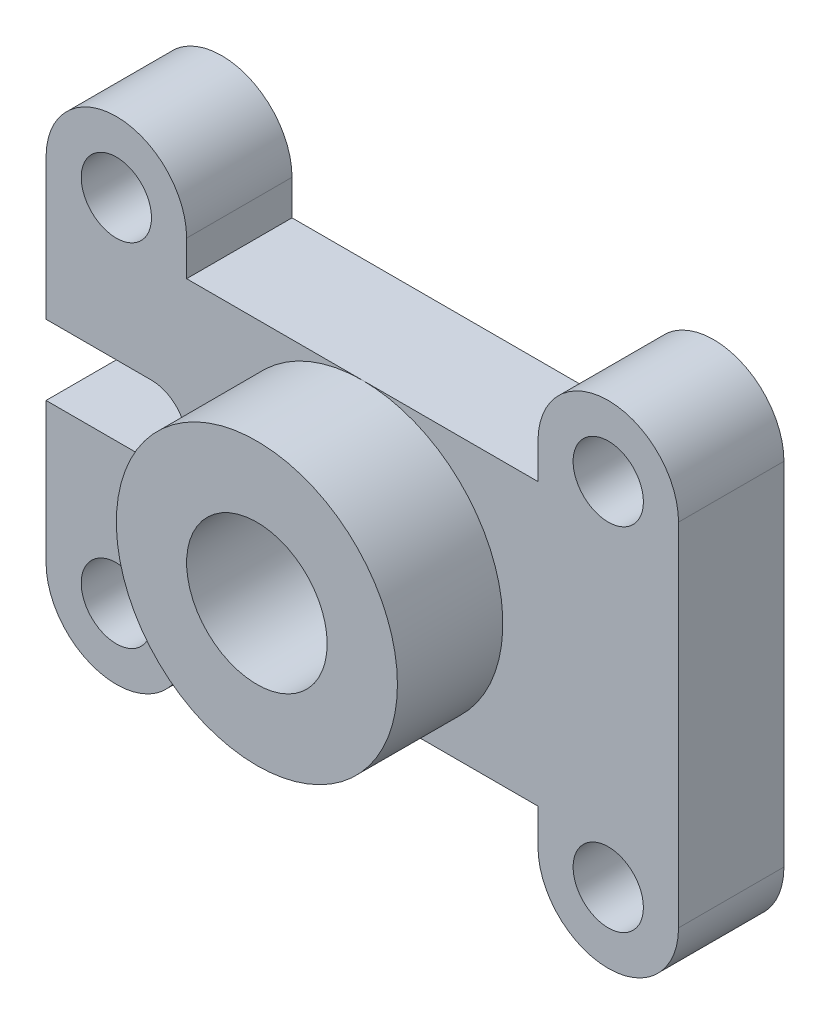
ISO-10303-21;
HEADER;
FILE_DESCRIPTION(('STEP AP214'),'2;1');
FILE_NAME('part.step','',(''),(''),'','','');
FILE_SCHEMA(('AUTOMOTIVE_DESIGN { 1 0 10303 214 1 1 1 1 }'));
ENDSEC;
DATA;
#1=APPLICATION_CONTEXT('core data for automotive mechanical design processes');
#2=APPLICATION_PROTOCOL_DEFINITION('international standard','automotive_design',2000,#1);
#3=PRODUCT_CONTEXT('',#1,'mechanical');
#4=PRODUCT('Part','Part','',(#3));
#5=PRODUCT_RELATED_PRODUCT_CATEGORY('part','',(#4));
#6=PRODUCT_DEFINITION_FORMATION('','',#4);
#7=PRODUCT_DEFINITION_CONTEXT('part definition',#1,'design');
#8=PRODUCT_DEFINITION('design','',#6,#7);
#9=PRODUCT_DEFINITION_SHAPE('','',#8);
#10=(LENGTH_UNIT() NAMED_UNIT(*) SI_UNIT(.MILLI.,.METRE.));
#11=(NAMED_UNIT(*) PLANE_ANGLE_UNIT() SI_UNIT($,.RADIAN.));
#12=(NAMED_UNIT(*) SI_UNIT($,.STERADIAN.) SOLID_ANGLE_UNIT());
#13=UNCERTAINTY_MEASURE_WITH_UNIT(LENGTH_MEASURE(1.E-05),#10,'distance_accuracy_value','');
#14=(GEOMETRIC_REPRESENTATION_CONTEXT(3) GLOBAL_UNCERTAINTY_ASSIGNED_CONTEXT((#13)) GLOBAL_UNIT_ASSIGNED_CONTEXT((#10,
#11,#12)) REPRESENTATION_CONTEXT('',''));
#15=CARTESIAN_POINT('',(0.,0.,0.));
#16=DIRECTION('',(0.,0.,1.));
#17=DIRECTION('',(1.,0.,0.));
#18=AXIS2_PLACEMENT_3D('',#15,#16,#17);
#19=CARTESIAN_POINT('',(-10.,0.,15.));
#20=DIRECTION('',(1.,0.,0.));
#21=DIRECTION('',(0.,1.,0.));
#22=AXIS2_PLACEMENT_3D('',#19,#20,#21);
#23=PLANE('',#22);
#24=DIRECTION('',(0.,-1.,0.));
#25=VECTOR('',#24,1.);
#26=CARTESIAN_POINT('',(-10.,0.,15.));
#27=LINE('',#26,#25);
#28=CARTESIAN_POINT('',(-10.,20.,15.));
#29=VERTEX_POINT('',#28);
#30=CARTESIAN_POINT('',(-10.,0.,15.));
#31=VERTEX_POINT('',#30);
#32=EDGE_CURVE('E262',#29,#31,#27,.T.);
#33=ORIENTED_EDGE('',*,*,#32,.F.);
#34=DIRECTION('',(0.,0.,1.));
#35=VECTOR('',#34,1.);
#36=CARTESIAN_POINT('',(-10.,20.,0.));
#37=LINE('',#36,#35);
#38=CARTESIAN_POINT('',(-10.,20.,0.));
#39=VERTEX_POINT('',#38);
#40=EDGE_CURVE('E197',#39,#29,#37,.T.);
#41=ORIENTED_EDGE('',*,*,#40,.F.);
#42=DIRECTION('',(0.,-1.,0.));
#43=VECTOR('',#42,1.);
#44=CARTESIAN_POINT('',(-10.,0.,0.));
#45=LINE('',#44,#43);
#46=CARTESIAN_POINT('',(-10.,0.,0.));
#47=VERTEX_POINT('',#46);
#48=EDGE_CURVE('E289',#39,#47,#45,.T.);
#49=ORIENTED_EDGE('',*,*,#48,.T.);
#50=DIRECTION('',(0.,0.,-1.));
#51=VECTOR('',#50,1.);
#52=CARTESIAN_POINT('',(-10.,0.,15.));
#53=LINE('',#52,#51);
#54=EDGE_CURVE('E322',#31,#47,#53,.T.);
#55=ORIENTED_EDGE('',*,*,#54,.F.);
#56=EDGE_LOOP('',(#33,#41,#49,#55));
#57=FACE_BOUND('',#56,.T.);
#58=ADVANCED_FACE('F50',(#57),#23,.F.);
#59=CARTESIAN_POINT('',(0.,0.,15.));
#60=DIRECTION('',(0.,0.,1.));
#61=DIRECTION('',(1.,0.,0.));
#62=AXIS2_PLACEMENT_3D('',#59,#60,#61);
#63=PLANE('',#62);
#64=DIRECTION('',(1.,0.,0.));
#65=VECTOR('',#64,1.);
#66=CARTESIAN_POINT('',(5.,20.,15.));
#67=LINE('',#66,#65);
#68=CARTESIAN_POINT('',(5.,20.,15.));
#69=VERTEX_POINT('',#68);
#70=EDGE_CURVE('E190',#29,#69,#67,.T.);
#71=ORIENTED_EDGE('',*,*,#70,.F.);
#72=ORIENTED_EDGE('',*,*,#32,.T.);
#73=CARTESIAN_POINT('',(0.,0.,15.));
#74=DIRECTION('',(0.,0.,1.));
#75=DIRECTION('',(1.,0.,0.));
#76=AXIS2_PLACEMENT_3D('',#73,#74,#75);
#77=CIRCLE('',#76,10.);
#78=CARTESIAN_POINT('',(10.,0.,15.));
#79=VERTEX_POINT('',#78);
#80=EDGE_CURVE('E268',#31,#79,#77,.T.);
#81=ORIENTED_EDGE('',*,*,#80,.T.);
#82=DIRECTION('',(0.,1.,0.));
#83=VECTOR('',#82,1.);
#84=CARTESIAN_POINT('',(10.,0.,15.));
#85=LINE('',#84,#83);
#86=CARTESIAN_POINT('',(10.,5.,15.));
#87=VERTEX_POINT('',#86);
#88=EDGE_CURVE('E269',#79,#87,#85,.T.);
#89=ORIENTED_EDGE('',*,*,#88,.T.);
#90=DIRECTION('',(-1.,0.,0.));
#91=VECTOR('',#90,1.);
#92=CARTESIAN_POINT('',(10.,5.,15.));
#93=LINE('',#92,#91);
#94=CARTESIAN_POINT('',(35.,5.00000000000001,15.));
#95=VERTEX_POINT('',#94);
#96=EDGE_CURVE('E245',#95,#87,#93,.T.);
#97=ORIENTED_EDGE('',*,*,#96,.F.);
#98=CARTESIAN_POINT('',(35.,25.,15.));
#99=DIRECTION('',(0.,0.,1.));
#100=DIRECTION('',(1.,0.,0.));
#101=AXIS2_PLACEMENT_3D('',#98,#99,#100);
#102=CIRCLE('',#101,20.);
#103=CARTESIAN_POINT('',(35.,45.,15.));
#104=VERTEX_POINT('',#103);
#105=EDGE_CURVE('E60',#104,#95,#102,.T.);
#106=ORIENTED_EDGE('',*,*,#105,.F.);
#107=DIRECTION('',(1.,0.,0.));
#108=VECTOR('',#107,1.);
#109=CARTESIAN_POINT('',(60.,45.,15.));
#110=LINE('',#109,#108);
#111=CARTESIAN_POINT('',(10.,45.,15.));
#112=VERTEX_POINT('',#111);
#113=EDGE_CURVE('E249',#112,#104,#110,.T.);
#114=ORIENTED_EDGE('',*,*,#113,.F.);
#115=DIRECTION('',(0.,1.,0.));
#116=VECTOR('',#115,1.);
#117=CARTESIAN_POINT('',(10.,0.,15.));
#118=LINE('',#117,#116);
#119=CARTESIAN_POINT('',(10.,50.,15.));
#120=VERTEX_POINT('',#119);
#121=EDGE_CURVE('E256',#112,#120,#118,.T.);
#122=ORIENTED_EDGE('',*,*,#121,.T.);
#123=CARTESIAN_POINT('',(0.,50.,15.));
#124=DIRECTION('',(0.,0.,1.));
#125=DIRECTION('',(1.,0.,0.));
#126=AXIS2_PLACEMENT_3D('',#123,#124,#125);
#127=CIRCLE('',#126,10.);
#128=CARTESIAN_POINT('',(-10.,50.,15.));
#129=VERTEX_POINT('',#128);
#130=EDGE_CURVE('E261',#120,#129,#127,.T.);
#131=ORIENTED_EDGE('',*,*,#130,.T.);
#132=CARTESIAN_POINT('',(-10.,30.,15.));
#133=VERTEX_POINT('',#132);
#134=EDGE_CURVE('E264',#129,#133,#27,.T.);
#135=ORIENTED_EDGE('',*,*,#134,.T.);
#136=DIRECTION('',(-1.,0.,0.));
#137=VECTOR('',#136,1.);
#138=CARTESIAN_POINT('',(5.,30.,15.));
#139=LINE('',#138,#137);
#140=CARTESIAN_POINT('',(5.,30.,15.));
#141=VERTEX_POINT('',#140);
#142=EDGE_CURVE('E188',#141,#133,#139,.T.);
#143=ORIENTED_EDGE('',*,*,#142,.F.);
#144=CARTESIAN_POINT('',(5.,25.,15.));
#145=DIRECTION('',(0.,0.,1.));
#146=DIRECTION('',(1.,0.,0.));
#147=AXIS2_PLACEMENT_3D('',#144,#145,#146);
#148=CIRCLE('',#147,5.);
#149=EDGE_CURVE('E174',#69,#141,#148,.T.);
#150=ORIENTED_EDGE('',*,*,#149,.F.);
#151=EDGE_LOOP('',(#71,#72,#81,#89,#97,#106,#114,#122,#131,#135,#143,#150));
#152=FACE_BOUND('',#151,.T.);
#153=CARTESIAN_POINT('',(0.,49.9999999999999,15.));
#154=DIRECTION('',(0.,0.,1.));
#155=DIRECTION('',(1.,0.,0.));
#156=AXIS2_PLACEMENT_3D('',#153,#154,#155);
#157=CIRCLE('',#156,5.);
#158=CARTESIAN_POINT('',(5.,49.9999999999999,15.));
#159=VERTEX_POINT('',#158);
#160=EDGE_CURVE('E198',#159,#159,#157,.T.);
#161=ORIENTED_EDGE('',*,*,#160,.F.);
#162=EDGE_LOOP('',(#161));
#163=FACE_BOUND('',#162,.T.);
#164=CARTESIAN_POINT('',(0.,0.,15.));
#165=DIRECTION('',(0.,0.,1.));
#166=DIRECTION('',(1.,0.,0.));
#167=AXIS2_PLACEMENT_3D('',#164,#165,#166);
#168=CIRCLE('',#167,5.);
#169=CARTESIAN_POINT('',(5.,0.,15.));
#170=VERTEX_POINT('',#169);
#171=EDGE_CURVE('E215',#170,#170,#168,.T.);
#172=ORIENTED_EDGE('',*,*,#171,.F.);
#173=EDGE_LOOP('',(#172));
#174=FACE_BOUND('',#173,.T.);
#175=ADVANCED_FACE('F342',(#152,#163,#174),#63,.T.);
#176=CARTESIAN_POINT('',(10.,0.,15.));
#177=DIRECTION('',(-1.,0.,0.));
#178=DIRECTION('',(0.,0.,1.));
#179=AXIS2_PLACEMENT_3D('',#176,#177,#178);
#180=PLANE('',#179);
#181=DIRECTION('',(0.,0.,-1.));
#182=VECTOR('',#181,1.);
#183=CARTESIAN_POINT('',(10.,5.,0.));
#184=LINE('',#183,#182);
#185=CARTESIAN_POINT('',(10.,5.,0.));
#186=VERTEX_POINT('',#185);
#187=EDGE_CURVE('E231',#87,#186,#184,.T.);
#188=ORIENTED_EDGE('',*,*,#187,.F.);
#189=ORIENTED_EDGE('',*,*,#88,.F.);
#190=DIRECTION('',(0.,0.,-1.));
#191=VECTOR('',#190,1.);
#192=CARTESIAN_POINT('',(10.,0.,15.));
#193=LINE('',#192,#191);
#194=CARTESIAN_POINT('',(10.,0.,0.));
#195=VERTEX_POINT('',#194);
#196=EDGE_CURVE('E319',#79,#195,#193,.T.);
#197=ORIENTED_EDGE('',*,*,#196,.T.);
#198=DIRECTION('',(0.,1.,0.));
#199=VECTOR('',#198,1.);
#200=CARTESIAN_POINT('',(10.,0.,0.));
#201=LINE('',#200,#199);
#202=EDGE_CURVE('E294',#195,#186,#201,.T.);
#203=ORIENTED_EDGE('',*,*,#202,.T.);
#204=EDGE_LOOP('',(#188,#189,#197,#203));
#205=FACE_BOUND('',#204,.T.);
#206=ADVANCED_FACE('F391',(#205),#180,.F.);
#207=CARTESIAN_POINT('',(60.,0.,15.));
#208=DIRECTION('',(-1.,0.,0.));
#209=DIRECTION('',(0.,0.,1.));
#210=AXIS2_PLACEMENT_3D('',#207,#208,#209);
#211=PLANE('',#210);
#212=DIRECTION('',(0.,1.,0.));
#213=VECTOR('',#212,1.);
#214=CARTESIAN_POINT('',(60.,0.,15.));
#215=LINE('',#214,#213);
#216=CARTESIAN_POINT('',(60.,0.,15.));
#217=VERTEX_POINT('',#216);
#218=CARTESIAN_POINT('',(60.,5.00000000000001,15.));
#219=VERTEX_POINT('',#218);
#220=EDGE_CURVE('E271',#217,#219,#215,.T.);
#221=ORIENTED_EDGE('',*,*,#220,.T.);
#222=DIRECTION('',(0.,0.,1.));
#223=VECTOR('',#222,1.);
#224=CARTESIAN_POINT('',(60.,5.00000000000001,15.));
#225=LINE('',#224,#223);
#226=CARTESIAN_POINT('',(60.,5.00000000000001,0.));
#227=VERTEX_POINT('',#226);
#228=EDGE_CURVE('E239',#227,#219,#225,.T.);
#229=ORIENTED_EDGE('',*,*,#228,.F.);
#230=DIRECTION('',(0.,1.,0.));
#231=VECTOR('',#230,1.);
#232=CARTESIAN_POINT('',(60.,0.,0.));
#233=LINE('',#232,#231);
#234=CARTESIAN_POINT('',(60.,0.,0.));
#235=VERTEX_POINT('',#234);
#236=EDGE_CURVE('E296',#235,#227,#233,.T.);
#237=ORIENTED_EDGE('',*,*,#236,.F.);
#238=DIRECTION('',(0.,0.,-1.));
#239=VECTOR('',#238,1.);
#240=CARTESIAN_POINT('',(60.,0.,15.));
#241=LINE('',#240,#239);
#242=EDGE_CURVE('E317',#217,#235,#241,.T.);
#243=ORIENTED_EDGE('',*,*,#242,.F.);
#244=EDGE_LOOP('',(#221,#229,#237,#243));
#245=FACE_BOUND('',#244,.T.);
#246=ADVANCED_FACE('F366',(#245),#211,.T.);
#247=CARTESIAN_POINT('',(10.,0.,15.));
#248=DIRECTION('',(-1.,0.,0.));
#249=DIRECTION('',(0.,0.,1.));
#250=AXIS2_PLACEMENT_3D('',#247,#248,#249);
#251=PLANE('',#250);
#252=DIRECTION('',(0.,0.,1.));
#253=VECTOR('',#252,1.);
#254=CARTESIAN_POINT('',(10.,45.,15.));
#255=LINE('',#254,#253);
#256=CARTESIAN_POINT('',(10.,45.,0.));
#257=VERTEX_POINT('',#256);
#258=EDGE_CURVE('E246',#257,#112,#255,.T.);
#259=ORIENTED_EDGE('',*,*,#258,.F.);
#260=DIRECTION('',(0.,1.,0.));
#261=VECTOR('',#260,1.);
#262=CARTESIAN_POINT('',(10.,0.,0.));
#263=LINE('',#262,#261);
#264=CARTESIAN_POINT('',(10.,50.,0.));
#265=VERTEX_POINT('',#264);
#266=EDGE_CURVE('E259',#257,#265,#263,.T.);
#267=ORIENTED_EDGE('',*,*,#266,.T.);
#268=DIRECTION('',(0.,0.,-1.));
#269=VECTOR('',#268,1.);
#270=CARTESIAN_POINT('',(10.,50.,15.));
#271=LINE('',#270,#269);
#272=EDGE_CURVE('E51',#120,#265,#271,.T.);
#273=ORIENTED_EDGE('',*,*,#272,.F.);
#274=ORIENTED_EDGE('',*,*,#121,.F.);
#275=EDGE_LOOP('',(#259,#267,#273,#274));
#276=FACE_BOUND('',#275,.T.);
#277=ADVANCED_FACE('F47',(#276),#251,.F.);
#278=CARTESIAN_POINT('',(60.,0.,15.));
#279=DIRECTION('',(1.,0.,0.));
#280=DIRECTION('',(0.,0.,-1.));
#281=AXIS2_PLACEMENT_3D('',#278,#279,#280);
#282=PLANE('',#281);
#283=DIRECTION('',(0.,0.,-1.));
#284=VECTOR('',#283,1.);
#285=CARTESIAN_POINT('',(60.,45.,0.));
#286=LINE('',#285,#284);
#287=CARTESIAN_POINT('',(60.,45.,15.));
#288=VERTEX_POINT('',#287);
#289=CARTESIAN_POINT('',(60.,45.,0.));
#290=VERTEX_POINT('',#289);
#291=EDGE_CURVE('E255',#288,#290,#286,.T.);
#292=ORIENTED_EDGE('',*,*,#291,.F.);
#293=DIRECTION('',(0.,-1.,0.));
#294=VECTOR('',#293,1.);
#295=CARTESIAN_POINT('',(60.,0.,15.));
#296=LINE('',#295,#294);
#297=CARTESIAN_POINT('',(60.,50.,15.));
#298=VERTEX_POINT('',#297);
#299=EDGE_CURVE('E283',#298,#288,#296,.T.);
#300=ORIENTED_EDGE('',*,*,#299,.F.);
#301=DIRECTION('',(0.,0.,-1.));
#302=VECTOR('',#301,1.);
#303=CARTESIAN_POINT('',(60.,50.,15.));
#304=LINE('',#303,#302);
#305=CARTESIAN_POINT('',(60.,50.,0.));
#306=VERTEX_POINT('',#305);
#307=EDGE_CURVE('E286',#298,#306,#304,.T.);
#308=ORIENTED_EDGE('',*,*,#307,.T.);
#309=DIRECTION('',(0.,-1.,0.));
#310=VECTOR('',#309,1.);
#311=CARTESIAN_POINT('',(60.,0.,0.));
#312=LINE('',#311,#310);
#313=EDGE_CURVE('E265',#306,#290,#312,.T.);
#314=ORIENTED_EDGE('',*,*,#313,.T.);
#315=EDGE_LOOP('',(#292,#300,#308,#314));
#316=FACE_BOUND('',#315,.T.);
#317=ADVANCED_FACE('F351',(#316),#282,.F.);
#318=CARTESIAN_POINT('',(0.,50.,15.));
#319=DIRECTION('',(0.,0.,-1.));
#320=DIRECTION('',(-1.,0.,0.));
#321=AXIS2_PLACEMENT_3D('',#318,#319,#320);
#322=CYLINDRICAL_SURFACE('',#321,10.);
#323=CARTESIAN_POINT('',(0.,50.,0.));
#324=DIRECTION('',(0.,0.,1.));
#325=DIRECTION('',(1.,0.,0.));
#326=AXIS2_PLACEMENT_3D('',#323,#324,#325);
#327=CIRCLE('',#326,10.);
#328=CARTESIAN_POINT('',(-10.,50.,0.));
#329=VERTEX_POINT('',#328);
#330=EDGE_CURVE('E288',#265,#329,#327,.T.);
#331=ORIENTED_EDGE('',*,*,#330,.T.);
#332=DIRECTION('',(0.,0.,-1.));
#333=VECTOR('',#332,1.);
#334=CARTESIAN_POINT('',(-10.,50.,15.));
#335=LINE('',#334,#333);
#336=EDGE_CURVE('E324',#129,#329,#335,.T.);
#337=ORIENTED_EDGE('',*,*,#336,.F.);
#338=ORIENTED_EDGE('',*,*,#130,.F.);
#339=ORIENTED_EDGE('',*,*,#272,.T.);
#340=EDGE_LOOP('',(#331,#337,#338,#339));
#341=FACE_BOUND('',#340,.T.);
#342=ADVANCED_FACE('F335',(#341),#322,.T.);
#343=CARTESIAN_POINT('',(-10.,30.,0.));
#344=VERTEX_POINT('',#343);
#345=EDGE_CURVE('E293',#329,#344,#45,.T.);
#346=ORIENTED_EDGE('',*,*,#345,.T.);
#347=DIRECTION('',(0.,0.,1.));
#348=VECTOR('',#347,1.);
#349=CARTESIAN_POINT('',(-10.,30.,0.));
#350=LINE('',#349,#348);
#351=EDGE_CURVE('E61',#344,#133,#350,.T.);
#352=ORIENTED_EDGE('',*,*,#351,.T.);
#353=ORIENTED_EDGE('',*,*,#134,.F.);
#354=ORIENTED_EDGE('',*,*,#336,.T.);
#355=EDGE_LOOP('',(#346,#352,#353,#354));
#356=FACE_BOUND('',#355,.T.);
#357=ADVANCED_FACE('F336',(#356),#23,.F.);
#358=CARTESIAN_POINT('',(0.,0.,15.));
#359=DIRECTION('',(0.,0.,-1.));
#360=DIRECTION('',(-1.,0.,0.));
#361=AXIS2_PLACEMENT_3D('',#358,#359,#360);
#362=CYLINDRICAL_SURFACE('',#361,10.);
#363=CARTESIAN_POINT('',(0.,0.,0.));
#364=DIRECTION('',(0.,0.,1.));
#365=DIRECTION('',(1.,0.,0.));
#366=AXIS2_PLACEMENT_3D('',#363,#364,#365);
#367=CIRCLE('',#366,10.);
#368=EDGE_CURVE('E291',#47,#195,#367,.T.);
#369=ORIENTED_EDGE('',*,*,#368,.T.);
#370=ORIENTED_EDGE('',*,*,#196,.F.);
#371=ORIENTED_EDGE('',*,*,#80,.F.);
#372=ORIENTED_EDGE('',*,*,#54,.T.);
#373=EDGE_LOOP('',(#369,#370,#371,#372));
#374=FACE_BOUND('',#373,.T.);
#375=ADVANCED_FACE('F372',(#374),#362,.T.);
#376=CARTESIAN_POINT('',(70.,0.,15.));
#377=DIRECTION('',(0.,0.,-1.));
#378=DIRECTION('',(-1.,0.,0.));
#379=AXIS2_PLACEMENT_3D('',#376,#377,#378);
#380=CYLINDRICAL_SURFACE('',#379,10.);
#381=CARTESIAN_POINT('',(70.,0.,0.));
#382=DIRECTION('',(0.,0.,1.));
#383=DIRECTION('',(1.,0.,0.));
#384=AXIS2_PLACEMENT_3D('',#381,#382,#383);
#385=CIRCLE('',#384,10.);
#386=CARTESIAN_POINT('',(80.,0.,0.));
#387=VERTEX_POINT('',#386);
#388=EDGE_CURVE('E301',#235,#387,#385,.T.);
#389=ORIENTED_EDGE('',*,*,#388,.T.);
#390=DIRECTION('',(0.,0.,-1.));
#391=VECTOR('',#390,1.);
#392=CARTESIAN_POINT('',(80.,0.,15.));
#393=LINE('',#392,#391);
#394=CARTESIAN_POINT('',(80.,0.,15.));
#395=VERTEX_POINT('',#394);
#396=EDGE_CURVE('E313',#395,#387,#393,.T.);
#397=ORIENTED_EDGE('',*,*,#396,.F.);
#398=CARTESIAN_POINT('',(70.,0.,15.));
#399=DIRECTION('',(0.,0.,1.));
#400=DIRECTION('',(1.,0.,0.));
#401=AXIS2_PLACEMENT_3D('',#398,#399,#400);
#402=CIRCLE('',#401,10.);
#403=EDGE_CURVE('E277',#217,#395,#402,.T.);
#404=ORIENTED_EDGE('',*,*,#403,.F.);
#405=ORIENTED_EDGE('',*,*,#242,.T.);
#406=EDGE_LOOP('',(#389,#397,#404,#405));
#407=FACE_BOUND('',#406,.T.);
#408=ADVANCED_FACE('F375',(#407),#380,.T.);
#409=CARTESIAN_POINT('',(80.,0.,15.));
#410=DIRECTION('',(1.,0.,0.));
#411=DIRECTION('',(0.,0.,-1.));
#412=AXIS2_PLACEMENT_3D('',#409,#410,#411);
#413=PLANE('',#412);
#414=DIRECTION('',(0.,-1.,0.));
#415=VECTOR('',#414,1.);
#416=CARTESIAN_POINT('',(80.,0.,0.));
#417=LINE('',#416,#415);
#418=CARTESIAN_POINT('',(80.,50.,0.));
#419=VERTEX_POINT('',#418);
#420=EDGE_CURVE('E302',#419,#387,#417,.T.);
#421=ORIENTED_EDGE('',*,*,#420,.F.);
#422=DIRECTION('',(0.,0.,-1.));
#423=VECTOR('',#422,1.);
#424=CARTESIAN_POINT('',(80.,50.,15.));
#425=LINE('',#424,#423);
#426=CARTESIAN_POINT('',(80.,50.,15.));
#427=VERTEX_POINT('',#426);
#428=EDGE_CURVE('E315',#427,#419,#425,.T.);
#429=ORIENTED_EDGE('',*,*,#428,.F.);
#430=DIRECTION('',(0.,-1.,0.));
#431=VECTOR('',#430,1.);
#432=CARTESIAN_POINT('',(80.,0.,15.));
#433=LINE('',#432,#431);
#434=EDGE_CURVE('E279',#427,#395,#433,.T.);
#435=ORIENTED_EDGE('',*,*,#434,.T.);
#436=ORIENTED_EDGE('',*,*,#396,.T.);
#437=EDGE_LOOP('',(#421,#429,#435,#436));
#438=FACE_BOUND('',#437,.T.);
#439=ADVANCED_FACE('F360',(#438),#413,.T.);
#440=CARTESIAN_POINT('',(70.,50.,15.));
#441=DIRECTION('',(0.,0.,-1.));
#442=DIRECTION('',(-1.,0.,0.));
#443=AXIS2_PLACEMENT_3D('',#440,#441,#442);
#444=CYLINDRICAL_SURFACE('',#443,10.);
#445=CARTESIAN_POINT('',(70.,50.,0.));
#446=DIRECTION('',(0.,0.,1.));
#447=DIRECTION('',(1.,0.,0.));
#448=AXIS2_PLACEMENT_3D('',#445,#446,#447);
#449=CIRCLE('',#448,10.);
#450=EDGE_CURVE('E310',#419,#306,#449,.T.);
#451=ORIENTED_EDGE('',*,*,#450,.T.);
#452=ORIENTED_EDGE('',*,*,#307,.F.);
#453=CARTESIAN_POINT('',(70.,50.,15.));
#454=DIRECTION('',(0.,0.,1.));
#455=DIRECTION('',(1.,0.,0.));
#456=AXIS2_PLACEMENT_3D('',#453,#454,#455);
#457=CIRCLE('',#456,10.);
#458=EDGE_CURVE('E281',#427,#298,#457,.T.);
#459=ORIENTED_EDGE('',*,*,#458,.F.);
#460=ORIENTED_EDGE('',*,*,#428,.T.);
#461=EDGE_LOOP('',(#451,#452,#459,#460));
#462=FACE_BOUND('',#461,.T.);
#463=ADVANCED_FACE('F358',(#462),#444,.T.);
#464=CARTESIAN_POINT('',(70.,0.,15.));
#465=DIRECTION('',(0.,0.,1.));
#466=DIRECTION('',(1.,0.,0.));
#467=AXIS2_PLACEMENT_3D('',#464,#465,#466);
#468=CIRCLE('',#467,5.);
#469=CARTESIAN_POINT('',(75.,0.,15.));
#470=VERTEX_POINT('',#469);
#471=EDGE_CURVE('E207',#470,#470,#468,.T.);
#472=ORIENTED_EDGE('',*,*,#471,.F.);
#473=EDGE_LOOP('',(#472));
#474=FACE_BOUND('',#473,.T.);
#475=CARTESIAN_POINT('',(70.,50.,15.));
#476=DIRECTION('',(0.,0.,1.));
#477=DIRECTION('',(1.,0.,0.));
#478=AXIS2_PLACEMENT_3D('',#475,#476,#477);
#479=CIRCLE('',#478,5.00000000000001);
#480=CARTESIAN_POINT('',(75.,50.,15.));
#481=VERTEX_POINT('',#480);
#482=EDGE_CURVE('E204',#481,#481,#479,.T.);
#483=ORIENTED_EDGE('',*,*,#482,.F.);
#484=EDGE_LOOP('',(#483));
#485=FACE_BOUND('',#484,.T.);
#486=EDGE_CURVE('E11',#95,#104,#102,.T.);
#487=ORIENTED_EDGE('',*,*,#486,.F.);
#488=EDGE_CURVE('E243',#219,#95,#93,.T.);
#489=ORIENTED_EDGE('',*,*,#488,.F.);
#490=ORIENTED_EDGE('',*,*,#220,.F.);
#491=ORIENTED_EDGE('',*,*,#403,.T.);
#492=ORIENTED_EDGE('',*,*,#434,.F.);
#493=ORIENTED_EDGE('',*,*,#458,.T.);
#494=ORIENTED_EDGE('',*,*,#299,.T.);
#495=EDGE_CURVE('E248',#104,#288,#110,.T.);
#496=ORIENTED_EDGE('',*,*,#495,.F.);
#497=EDGE_LOOP('',(#487,#489,#490,#491,#492,#493,#494,#496));
#498=FACE_BOUND('',#497,.T.);
#499=ADVANCED_FACE('F371',(#474,#485,#498),#63,.T.);
#500=CARTESIAN_POINT('',(0.,0.,0.));
#501=DIRECTION('',(0.,0.,1.));
#502=DIRECTION('',(1.,0.,0.));
#503=AXIS2_PLACEMENT_3D('',#500,#501,#502);
#504=PLANE('',#503);
#505=CARTESIAN_POINT('',(0.,49.9999999999999,0.));
#506=DIRECTION('',(0.,0.,1.));
#507=DIRECTION('',(1.,0.,0.));
#508=AXIS2_PLACEMENT_3D('',#505,#506,#507);
#509=CIRCLE('',#508,5.);
#510=CARTESIAN_POINT('',(5.,49.9999999999999,0.));
#511=VERTEX_POINT('',#510);
#512=EDGE_CURVE('E213',#511,#511,#509,.T.);
#513=ORIENTED_EDGE('',*,*,#512,.T.);
#514=EDGE_LOOP('',(#513));
#515=FACE_BOUND('',#514,.T.);
#516=CARTESIAN_POINT('',(0.,0.,0.));
#517=DIRECTION('',(0.,0.,1.));
#518=DIRECTION('',(1.,0.,0.));
#519=AXIS2_PLACEMENT_3D('',#516,#517,#518);
#520=CIRCLE('',#519,5.);
#521=CARTESIAN_POINT('',(5.,0.,0.));
#522=VERTEX_POINT('',#521);
#523=EDGE_CURVE('E209',#522,#522,#520,.T.);
#524=ORIENTED_EDGE('',*,*,#523,.T.);
#525=EDGE_LOOP('',(#524));
#526=FACE_BOUND('',#525,.T.);
#527=CARTESIAN_POINT('',(70.,0.,0.));
#528=DIRECTION('',(0.,0.,1.));
#529=DIRECTION('',(1.,0.,0.));
#530=AXIS2_PLACEMENT_3D('',#527,#528,#529);
#531=CIRCLE('',#530,5.);
#532=CARTESIAN_POINT('',(75.,0.,0.));
#533=VERTEX_POINT('',#532);
#534=EDGE_CURVE('E205',#533,#533,#531,.T.);
#535=ORIENTED_EDGE('',*,*,#534,.T.);
#536=EDGE_LOOP('',(#535));
#537=FACE_BOUND('',#536,.T.);
#538=CARTESIAN_POINT('',(70.,50.,0.));
#539=DIRECTION('',(0.,0.,1.));
#540=DIRECTION('',(1.,0.,0.));
#541=AXIS2_PLACEMENT_3D('',#538,#539,#540);
#542=CIRCLE('',#541,5.00000000000001);
#543=CARTESIAN_POINT('',(75.,50.,0.));
#544=VERTEX_POINT('',#543);
#545=EDGE_CURVE('E219',#544,#544,#542,.T.);
#546=ORIENTED_EDGE('',*,*,#545,.T.);
#547=EDGE_LOOP('',(#546));
#548=FACE_BOUND('',#547,.T.);
#549=ORIENTED_EDGE('',*,*,#48,.F.);
#550=DIRECTION('',(1.,0.,0.));
#551=VECTOR('',#550,1.);
#552=CARTESIAN_POINT('',(5.,20.,0.));
#553=LINE('',#552,#551);
#554=CARTESIAN_POINT('',(5.,20.,0.));
#555=VERTEX_POINT('',#554);
#556=EDGE_CURVE('E180',#39,#555,#553,.T.);
#557=ORIENTED_EDGE('',*,*,#556,.T.);
#558=CARTESIAN_POINT('',(5.,25.,0.));
#559=DIRECTION('',(0.,0.,1.));
#560=DIRECTION('',(1.,0.,0.));
#561=AXIS2_PLACEMENT_3D('',#558,#559,#560);
#562=CIRCLE('',#561,5.);
#563=CARTESIAN_POINT('',(5.,30.,0.));
#564=VERTEX_POINT('',#563);
#565=EDGE_CURVE('E175',#555,#564,#562,.T.);
#566=ORIENTED_EDGE('',*,*,#565,.T.);
#567=DIRECTION('',(-1.,0.,0.));
#568=VECTOR('',#567,1.);
#569=CARTESIAN_POINT('',(5.,30.,0.));
#570=LINE('',#569,#568);
#571=EDGE_CURVE('E177',#564,#344,#570,.T.);
#572=ORIENTED_EDGE('',*,*,#571,.T.);
#573=ORIENTED_EDGE('',*,*,#345,.F.);
#574=ORIENTED_EDGE('',*,*,#330,.F.);
#575=ORIENTED_EDGE('',*,*,#266,.F.);
#576=DIRECTION('',(-1.,0.,0.));
#577=VECTOR('',#576,1.);
#578=CARTESIAN_POINT('',(10.,45.,0.));
#579=LINE('',#578,#577);
#580=EDGE_CURVE('E253',#290,#257,#579,.T.);
#581=ORIENTED_EDGE('',*,*,#580,.F.);
#582=ORIENTED_EDGE('',*,*,#313,.F.);
#583=ORIENTED_EDGE('',*,*,#450,.F.);
#584=ORIENTED_EDGE('',*,*,#420,.T.);
#585=ORIENTED_EDGE('',*,*,#388,.F.);
#586=ORIENTED_EDGE('',*,*,#236,.T.);
#587=DIRECTION('',(1.,0.,0.));
#588=VECTOR('',#587,1.);
#589=CARTESIAN_POINT('',(60.,5.00000000000001,0.));
#590=LINE('',#589,#588);
#591=EDGE_CURVE('E238',#186,#227,#590,.T.);
#592=ORIENTED_EDGE('',*,*,#591,.F.);
#593=ORIENTED_EDGE('',*,*,#202,.F.);
#594=ORIENTED_EDGE('',*,*,#368,.F.);
#595=EDGE_LOOP('',(#549,#557,#566,#572,#573,#574,#575,#581,#582,#583,#584,#585,#586,#592,#593,#594));
#596=FACE_BOUND('',#595,.T.);
#597=ADVANCED_FACE('F187',(#515,#526,#537,#548,#596),#504,.F.);
#598=CARTESIAN_POINT('',(0.,45.,0.));
#599=DIRECTION('',(0.,-1.,0.));
#600=DIRECTION('',(0.,0.,-1.));
#601=AXIS2_PLACEMENT_3D('',#598,#599,#600);
#602=PLANE('',#601);
#603=ORIENTED_EDGE('',*,*,#258,.T.);
#604=ORIENTED_EDGE('',*,*,#113,.T.);
#605=ORIENTED_EDGE('',*,*,#495,.T.);
#606=ORIENTED_EDGE('',*,*,#291,.T.);
#607=ORIENTED_EDGE('',*,*,#580,.T.);
#608=EDGE_LOOP('',(#603,#604,#605,#606,#607));
#609=FACE_BOUND('',#608,.T.);
#610=ADVANCED_FACE('F343',(#609),#602,.F.);
#611=CARTESIAN_POINT('',(0.,5.,0.));
#612=DIRECTION('',(0.,1.,0.));
#613=DIRECTION('',(-1.,0.,0.));
#614=AXIS2_PLACEMENT_3D('',#611,#612,#613);
#615=PLANE('',#614);
#616=ORIENTED_EDGE('',*,*,#187,.T.);
#617=ORIENTED_EDGE('',*,*,#591,.T.);
#618=ORIENTED_EDGE('',*,*,#228,.T.);
#619=ORIENTED_EDGE('',*,*,#488,.T.);
#620=ORIENTED_EDGE('',*,*,#96,.T.);
#621=EDGE_LOOP('',(#616,#617,#618,#619,#620));
#622=FACE_BOUND('',#621,.T.);
#623=ADVANCED_FACE('F369',(#622),#615,.F.);
#624=CARTESIAN_POINT('',(35.,25.,30.));
#625=DIRECTION('',(0.,0.,-1.));
#626=DIRECTION('',(-1.,0.,0.));
#627=AXIS2_PLACEMENT_3D('',#624,#625,#626);
#628=CYLINDRICAL_SURFACE('',#627,20.);
#629=CARTESIAN_POINT('',(35.,25.,30.));
#630=DIRECTION('',(0.,0.,1.));
#631=DIRECTION('',(1.,0.,0.));
#632=AXIS2_PLACEMENT_3D('',#629,#630,#631);
#633=CIRCLE('',#632,20.);
#634=CARTESIAN_POINT('',(55.,25.,30.));
#635=VERTEX_POINT('',#634);
#636=EDGE_CURVE('E233',#635,#635,#633,.T.);
#637=ORIENTED_EDGE('',*,*,#636,.F.);
#638=EDGE_LOOP('',(#637));
#639=FACE_BOUND('',#638,.T.);
#640=ORIENTED_EDGE('',*,*,#105,.T.);
#641=ORIENTED_EDGE('',*,*,#486,.T.);
#642=EDGE_LOOP('',(#640,#641));
#643=FACE_BOUND('',#642,.T.);
#644=ADVANCED_FACE('F428',(#639,#643),#628,.T.);
#645=CARTESIAN_POINT('',(35.,25.,30.));
#646=DIRECTION('',(0.,0.,1.));
#647=DIRECTION('',(1.,0.,0.));
#648=AXIS2_PLACEMENT_3D('',#645,#646,#647);
#649=PLANE('',#648);
#650=CARTESIAN_POINT('',(35.,25.,30.));
#651=DIRECTION('',(0.,0.,1.));
#652=DIRECTION('',(1.,0.,0.));
#653=AXIS2_PLACEMENT_3D('',#650,#651,#652);
#654=CIRCLE('',#653,10.);
#655=CARTESIAN_POINT('',(45.,25.,30.));
#656=VERTEX_POINT('',#655);
#657=EDGE_CURVE('E223',#656,#656,#654,.T.);
#658=ORIENTED_EDGE('',*,*,#657,.F.);
#659=EDGE_LOOP('',(#658));
#660=FACE_BOUND('',#659,.T.);
#661=ORIENTED_EDGE('',*,*,#636,.T.);
#662=EDGE_LOOP('',(#661));
#663=FACE_BOUND('',#662,.T.);
#664=ADVANCED_FACE('F429',(#660,#663),#649,.T.);
#665=CARTESIAN_POINT('',(35.,25.,15.));
#666=DIRECTION('',(0.,0.,1.));
#667=DIRECTION('',(1.,0.,0.));
#668=AXIS2_PLACEMENT_3D('',#665,#666,#667);
#669=CYLINDRICAL_SURFACE('',#668,10.);
#670=CARTESIAN_POINT('',(35.,25.,15.));
#671=DIRECTION('',(0.,0.,1.));
#672=DIRECTION('',(1.,0.,0.));
#673=AXIS2_PLACEMENT_3D('',#670,#671,#672);
#674=CIRCLE('',#673,10.);
#675=CARTESIAN_POINT('',(45.,25.,15.));
#676=VERTEX_POINT('',#675);
#677=EDGE_CURVE('E228',#676,#676,#674,.T.);
#678=ORIENTED_EDGE('',*,*,#677,.F.);
#679=EDGE_LOOP('',(#678));
#680=FACE_BOUND('',#679,.T.);
#681=ORIENTED_EDGE('',*,*,#657,.T.);
#682=EDGE_LOOP('',(#681));
#683=FACE_BOUND('',#682,.T.);
#684=ADVANCED_FACE('F433',(#680,#683),#669,.F.);
#685=CARTESIAN_POINT('',(35.,25.,15.));
#686=DIRECTION('',(0.,0.,1.));
#687=DIRECTION('',(1.,0.,0.));
#688=AXIS2_PLACEMENT_3D('',#685,#686,#687);
#689=PLANE('',#688);
#690=ORIENTED_EDGE('',*,*,#677,.T.);
#691=EDGE_LOOP('',(#690));
#692=FACE_BOUND('',#691,.T.);
#693=ADVANCED_FACE('F440',(#692),#689,.T.);
#694=CARTESIAN_POINT('',(70.,50.,0.));
#695=DIRECTION('',(0.,0.,1.));
#696=DIRECTION('',(1.,0.,0.));
#697=AXIS2_PLACEMENT_3D('',#694,#695,#696);
#698=CYLINDRICAL_SURFACE('',#697,5.00000000000001);
#699=ORIENTED_EDGE('',*,*,#545,.F.);
#700=EDGE_LOOP('',(#699));
#701=FACE_BOUND('',#700,.T.);
#702=ORIENTED_EDGE('',*,*,#482,.T.);
#703=EDGE_LOOP('',(#702));
#704=FACE_BOUND('',#703,.T.);
#705=ADVANCED_FACE('F441',(#701,#704),#698,.F.);
#706=CARTESIAN_POINT('',(70.,0.,0.));
#707=DIRECTION('',(0.,0.,1.));
#708=DIRECTION('',(1.,0.,0.));
#709=AXIS2_PLACEMENT_3D('',#706,#707,#708);
#710=CYLINDRICAL_SURFACE('',#709,5.);
#711=ORIENTED_EDGE('',*,*,#534,.F.);
#712=EDGE_LOOP('',(#711));
#713=FACE_BOUND('',#712,.T.);
#714=ORIENTED_EDGE('',*,*,#471,.T.);
#715=EDGE_LOOP('',(#714));
#716=FACE_BOUND('',#715,.T.);
#717=ADVANCED_FACE('F444',(#713,#716),#710,.F.);
#718=CARTESIAN_POINT('',(0.,0.,0.));
#719=DIRECTION('',(0.,0.,1.));
#720=DIRECTION('',(1.,0.,0.));
#721=AXIS2_PLACEMENT_3D('',#718,#719,#720);
#722=CYLINDRICAL_SURFACE('',#721,5.);
#723=ORIENTED_EDGE('',*,*,#523,.F.);
#724=EDGE_LOOP('',(#723));
#725=FACE_BOUND('',#724,.T.);
#726=ORIENTED_EDGE('',*,*,#171,.T.);
#727=EDGE_LOOP('',(#726));
#728=FACE_BOUND('',#727,.T.);
#729=ADVANCED_FACE('F448',(#725,#728),#722,.F.);
#730=CARTESIAN_POINT('',(0.,49.9999999999999,0.));
#731=DIRECTION('',(0.,0.,1.));
#732=DIRECTION('',(1.,0.,0.));
#733=AXIS2_PLACEMENT_3D('',#730,#731,#732);
#734=CYLINDRICAL_SURFACE('',#733,5.);
#735=ORIENTED_EDGE('',*,*,#512,.F.);
#736=EDGE_LOOP('',(#735));
#737=FACE_BOUND('',#736,.T.);
#738=ORIENTED_EDGE('',*,*,#160,.T.);
#739=EDGE_LOOP('',(#738));
#740=FACE_BOUND('',#739,.T.);
#741=ADVANCED_FACE('F450',(#737,#740),#734,.F.);
#742=CARTESIAN_POINT('',(5.,25.,0.));
#743=DIRECTION('',(0.,0.,1.));
#744=DIRECTION('',(1.,0.,0.));
#745=AXIS2_PLACEMENT_3D('',#742,#743,#744);
#746=CYLINDRICAL_SURFACE('',#745,5.);
#747=ORIENTED_EDGE('',*,*,#149,.T.);
#748=DIRECTION('',(0.,0.,1.));
#749=VECTOR('',#748,1.);
#750=CARTESIAN_POINT('',(5.,30.,0.));
#751=LINE('',#750,#749);
#752=EDGE_CURVE('E169',#564,#141,#751,.T.);
#753=ORIENTED_EDGE('',*,*,#752,.F.);
#754=ORIENTED_EDGE('',*,*,#565,.F.);
#755=DIRECTION('',(0.,0.,1.));
#756=VECTOR('',#755,1.);
#757=CARTESIAN_POINT('',(5.,20.,0.));
#758=LINE('',#757,#756);
#759=EDGE_CURVE('E196',#555,#69,#758,.T.);
#760=ORIENTED_EDGE('',*,*,#759,.T.);
#761=EDGE_LOOP('',(#747,#753,#754,#760));
#762=FACE_BOUND('',#761,.T.);
#763=ADVANCED_FACE('F167',(#762),#746,.F.);
#764=CARTESIAN_POINT('',(5.,20.,0.));
#765=DIRECTION('',(0.,-1.,0.));
#766=DIRECTION('',(0.,0.,-1.));
#767=AXIS2_PLACEMENT_3D('',#764,#765,#766);
#768=PLANE('',#767);
#769=ORIENTED_EDGE('',*,*,#70,.T.);
#770=ORIENTED_EDGE('',*,*,#759,.F.);
#771=ORIENTED_EDGE('',*,*,#556,.F.);
#772=ORIENTED_EDGE('',*,*,#40,.T.);
#773=EDGE_LOOP('',(#769,#770,#771,#772));
#774=FACE_BOUND('',#773,.T.);
#775=ADVANCED_FACE('F459',(#774),#768,.F.);
#776=CARTESIAN_POINT('',(5.,30.,0.));
#777=DIRECTION('',(0.,1.,0.));
#778=DIRECTION('',(0.,0.,1.));
#779=AXIS2_PLACEMENT_3D('',#776,#777,#778);
#780=PLANE('',#779);
#781=ORIENTED_EDGE('',*,*,#142,.T.);
#782=ORIENTED_EDGE('',*,*,#351,.F.);
#783=ORIENTED_EDGE('',*,*,#571,.F.);
#784=ORIENTED_EDGE('',*,*,#752,.T.);
#785=EDGE_LOOP('',(#781,#782,#783,#784));
#786=FACE_BOUND('',#785,.T.);
#787=ADVANCED_FACE('F179',(#786),#780,.F.);
#788=CLOSED_SHELL('',(#58,#175,#206,#246,#277,#317,#342,#357,#375,#408,#439,#463,#499,#597,#610,
#623,#644,#664,#684,#693,#705,#717,#729,#741,#763,#775,#787));
#789=MANIFOLD_SOLID_BREP('B2',#788);
#790=ADVANCED_BREP_SHAPE_REPRESENTATION('',(#18,#789),#14);
#791=SHAPE_DEFINITION_REPRESENTATION(#9,#790);
ENDSEC;
END-ISO-10303-21;
